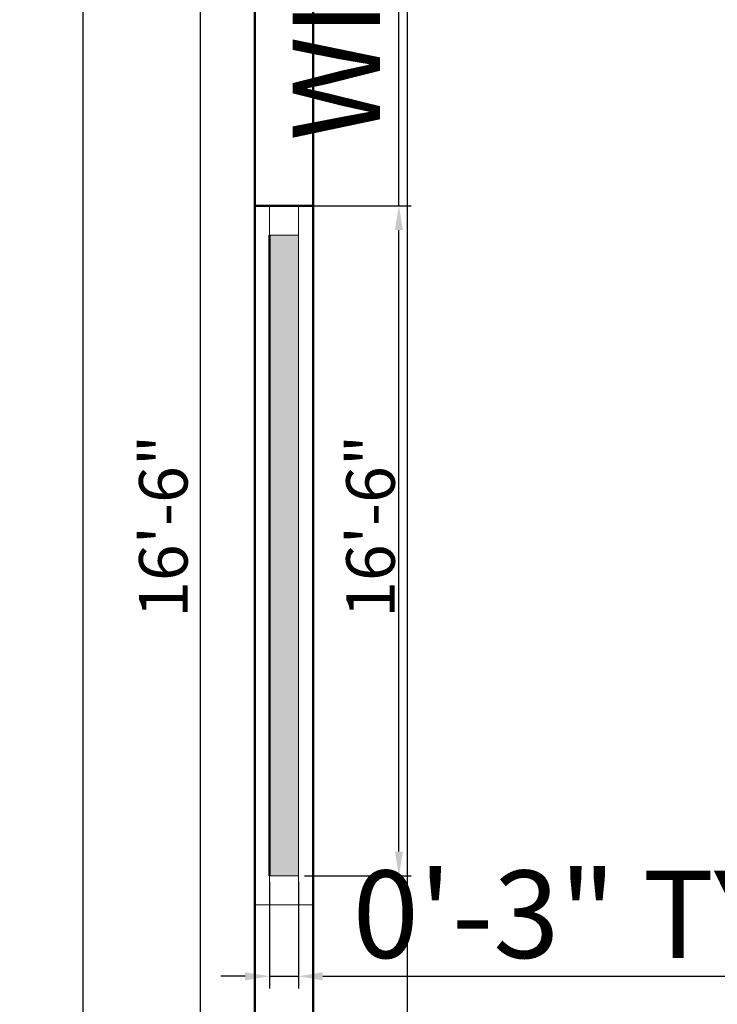
# Model space of a CAD drawing. Units: inches. Extents: x 3064 to 19385, y 846 to 15425.
# Tile 94 of 108: x 7502 to 7574, y 1032 to 1134. Entities that reach past the tile are written whole.
import ezdxf

# ---------------------------------------------------------------- set-up
doc = ezdxf.new("R2010")
doc.units = ezdxf.units.IN
for name, color, linetype, lineweight in [('A-ANNO-DIMS', 2, 'Continuous', 18), ('A-GLAZ', 4, 'Continuous', 18), ('A-WALL', 7, 'Continuous', 50)]:
    doc.layers.add(name, color=color, linetype=linetype, lineweight=lineweight)
doc.styles.get("Standard").update_dxf_attribs({"font": 'arial.ttf'})
doc.dimstyles.new('ISO-25', dxfattribs={"dimtxt": 9, "dimasz": 2.5, "dimexe": 1.25, "dimexo": 0.625, "dimtad": 1, "dimdec": 1, "dimlunit": 3, "dimtxsty": 'Standard', "dimcen": 2.5, "dimadec": 0, "dimazin": 0, "dimtfac": 1, "dimtdec": 1, "dimtmove": 0, "dimatfit": 3, "dimfxl": 1, "dimarcsym": 0})

# ---------------------------------------------------------------- blocks, each defined once
blk = doc.blocks.new('*D318')
at = {"layer": 'A-ANNO-DIMS', "color": 0, "lineweight": -2, "transparency": 16777216}
for p, q in [((7531.62, 1180.34), (7519.4, 1180.34)), ((7520.65, 984.84), (7520.65, 1177.84)), ((7531.62, 982.34), (7519.4, 982.34))]:
    blk.add_line(p, q, dxfattribs=at)
at = {"layer": 'A-ANNO-DIMS', "color": 0, "transparency": 16777216}
for points in [[(7520.23, 1177.84), (7521.06, 1177.84), (7520.65, 1180.34)], [(7520.23, 984.84), (7521.06, 984.84), (7520.65, 982.34)]]:
    blk.add_solid(points, dxfattribs=at)
at = {"layer": 'Defpoints', "color": 0, "transparency": 16777216}
for p in [(7520.65, 1180.34), (7532.25, 1180.34), (7532.25, 982.34)]:
    blk.add_point(p, dxfattribs=at)
at = {"layer": 'A-ANNO-DIMS', "color": 0, "transparency": 16777216, "insert": (7517.47, 1081.34), "char_height": 5, "attachment_point": 5, "rotation": 90}
blk.add_mtext('16\'-6"', dxfattribs=at)
blk = doc.blocks.new('*D324')
at = {"layer": 'A-ANNO-DIMS', "color": 0, "lineweight": -2, "transparency": 16777216}
for p, q in [((7525.62, 1396.34), (7507.31, 1396.34)), ((7508.56, 906.84), (7508.56, 1393.84)), ((7525.62, 904.34), (7507.31, 904.34))]:
    blk.add_line(p, q, dxfattribs=at)
at = {"layer": 'A-ANNO-DIMS', "color": 0, "transparency": 16777216}
for points in [[(7508.15, 1393.84), (7508.98, 1393.84), (7508.56, 1396.34)], [(7508.15, 906.84), (7508.98, 906.84), (7508.56, 904.34)]]:
    blk.add_solid(points, dxfattribs=at)
at = {"layer": 'Defpoints', "color": 0, "transparency": 16777216}
for p in [(7508.56, 1396.34), (7526.25, 1396.34), (7526.25, 904.34)]:
    blk.add_point(p, dxfattribs=at)
at = {"layer": 'A-ANNO-DIMS', "color": 0, "transparency": 16777216, "insert": (7505.43, 1150.34), "char_height": 5, "attachment_point": 5, "rotation": 90}
blk.add_mtext("41'", dxfattribs=at)
blk = doc.blocks.new('*D219')
at = {"layer": 'A-ANNO-DIMS', "color": 0, "lineweight": -2, "transparency": 16777216}
for p, q in [((7532.87, 1180.34), (7543.24, 1180.34)), ((7541.99, 984.84), (7541.99, 1177.84)), ((7532.87, 982.34), (7543.24, 982.34))]:
    blk.add_line(p, q, dxfattribs=at)
at = {"layer": 'A-ANNO-DIMS', "color": 0, "transparency": 16777216}
for points in [[(7541.58, 1177.84), (7542.41, 1177.84), (7541.99, 1180.34)], [(7541.58, 984.84), (7542.41, 984.84), (7541.99, 982.34)]]:
    blk.add_solid(points, dxfattribs=at)
at = {"layer": 'Defpoints', "color": 0, "transparency": 16777216}
for p in [(7532.25, 1180.34), (7541.99, 1180.34), (7532.25, 982.34)]:
    blk.add_point(p, dxfattribs=at)
at = {"layer": 'A-ANNO-DIMS', "color": 0, "transparency": 16777216, "insert": (7538.82, 1081.34), "char_height": 5, "attachment_point": 5, "rotation": 90}
blk.add_mtext('16\'-6"', dxfattribs=at)
blk = doc.blocks.new('WIN-1900')
blk.add_line((3, 0), (3, 66))
blk.add_lwpolyline([(3, 66), (0, 66), (0, 69), (3, 69)], close=True)
blk = doc.blocks.new('*D431')
at = {"layer": 'A-ANNO-DIMS', "color": 0, "lineweight": -2, "transparency": 16777216}
for p, q in [((7541.1, 1114.34), (7541.1, 1275.31)), ((7531.37, 1114.34), (7542.35, 1114.34)), ((7541.1, 1047.84), (7541.1, 1111.84)), ((7531.37, 1045.34), (7542.35, 1045.34))]:
    blk.add_line(p, q, dxfattribs=at)
at = {"layer": 'A-ANNO-DIMS', "color": 0, "transparency": 16777216}
for points in [[(7540.68, 1111.84), (7541.51, 1111.84), (7541.1, 1114.34)], [(7540.68, 1047.84), (7541.51, 1047.84), (7541.1, 1045.34)]]:
    blk.add_solid(points, dxfattribs=at)
at = {"layer": 'Defpoints', "color": 0, "transparency": 16777216}
for p in [(7530.75, 1114.34), (7541.1, 1114.34), (7530.75, 1045.34)]:
    blk.add_point(p, dxfattribs=at)
at = {"layer": 'A-ANNO-DIMS', "color": 0, "transparency": 16777216, "insert": (7535.81, 1196.07), "char_height": 9, "attachment_point": 5, "rotation": 90}
blk.add_mtext('WINDOW W1900 5\'-9" TYP.', dxfattribs=at)
blk = doc.blocks.new('*D432')
at = {"layer": 'A-ANNO-DIMS', "color": 0, "lineweight": -2, "transparency": 16777216}
for p, q in [((7527.75, 1044.71), (7527.75, 1033.74)), ((7530.75, 1044.71), (7530.75, 1033.74)), ((7525.25, 1034.99), (7522.75, 1034.99)), ((7527.75, 1034.99), (7530.75, 1034.99)), ((7533.25, 1034.99), (7591.86, 1034.99))]:
    blk.add_line(p, q, dxfattribs=at)
at = {"layer": 'A-ANNO-DIMS', "color": 0, "transparency": 16777216}
for points in [[(7525.25, 1035.41), (7525.25, 1034.57), (7527.75, 1034.99)], [(7533.25, 1035.41), (7533.25, 1034.57), (7530.75, 1034.99)]]:
    blk.add_solid(points, dxfattribs=at)
at = {"layer": 'Defpoints', "color": 0, "transparency": 16777216}
for p in [(7527.75, 1045.34), (7530.75, 1045.34), (7530.75, 1034.99)]:
    blk.add_point(p, dxfattribs=at)
at = {"layer": 'A-ANNO-DIMS', "color": 0, "transparency": 16777216, "insert": (7563.8, 1040.21), "char_height": 9, "attachment_point": 5}
blk.add_mtext('0\'-3" TYP.', dxfattribs=at)

msp = doc.modelspace()

# ---------------------------------------------------------------- hatches: boundary and pattern name
at = {"layer": 'A-GLAZ'}
h = msp.add_hatch(color=256, dxfattribs=at)
h.dxf.hatch_style = 1
h.paths.add_polyline_path([(7527.75, 1045.34), (7530.75, 1045.34), (7530.75, 1111.34), (7527.75, 1111.34)])

# ---------------------------------------------------------------- linework, layer by layer
msp.add_line((7532.25, 1042.34), (7526.25, 1042.34), dxfattribs=at)
msp.add_lwpolyline([(7530.75, 1042.34), (7527.75, 1042.34), (7527.75, 1045.34), (7530.75, 1045.34)], close=True, dxfattribs=at)
at = {"layer": 'A-WALL'}
for p, q in [((7526.25, 1396.34), (7526.25, 976.34)), ((7532.25, 1180.34), (7532.25, 982.34)), ((7532.25, 1114.34), (7526.25, 1114.34)), ((7527.75, 1045.34), (7527.75, 1111.34))]:
    msp.add_line(p, q, dxfattribs=at)

# ---------------------------------------------------------------- block references
at = {"layer": 'A-GLAZ'}
msp.add_blockref('WIN-1900', (7527.75, 1045.34), dxfattribs=at)

# ---------------------------------------------------------------- dimensions: what is measured, and where the dimension line sits
at = {"layer": 'A-ANNO-DIMS'}
for base, p1, p2, override, picture, middle in [((7508.56, 1396.34), (7526.25, 904.34), (7526.25, 1396.34), {"dimtxt": 5, "dimclrd": 0, "dimclre": 0, "dimclrt": 0}, '*D324', (7505.43, 1150.34)), ((7520.65, 1180.34), (7532.25, 982.34), (7532.25, 1180.34), {"dimtxt": 5, "dimclrd": 0, "dimclre": 0, "dimclrt": 0, "dimtmove": 1}, '*D318', (7517.47, 1081.34)), ((7541.99, 1180.34), (7532.25, 982.34), (7532.25, 1180.34), {"dimtxt": 5, "dimclrd": 0, "dimclre": 0, "dimclrt": 0}, '*D219', (7538.82, 1081.34))]:
    dim = msp.add_linear_dim(base=base, p1=p1, p2=p2, angle=90, dimstyle='ISO-25', override=override, dxfattribs=at)
    dim.commit()
    dim.dimension.update_dxf_attribs({"geometry": picture, "text_midpoint": middle})
dim = msp.add_linear_dim(base=(7541.1, 1114.34), p1=(7530.75, 1045.34), p2=(7530.75, 1114.34), angle=90, text='WINDOW W1900 <> TYP.', dimstyle='ISO-25', override={"dimdec": 1, "dimrnd": 0, "dimzin": 1, "dimlunit": 4, "dimfrac": 2}, dxfattribs=at)
dim.commit()
dim.dimension.update_dxf_attribs({"geometry": '*D431', "text_midpoint": (7535.81, 1196.07)})
dim = msp.add_linear_dim(base=(7530.75, 1034.99), p1=(7527.75, 1045.34), p2=(7530.75, 1045.34), text='<> TYP.', dimstyle='ISO-25', override={"dimdec": 1, "dimrnd": 0, "dimzin": 1, "dimlunit": 4, "dimfrac": 2}, dxfattribs=at)
dim.commit()
dim.dimension.update_dxf_attribs({"geometry": '*D432', "text_midpoint": (7563.8, 1040.21)})

doc.saveas('drawing.dxf')
